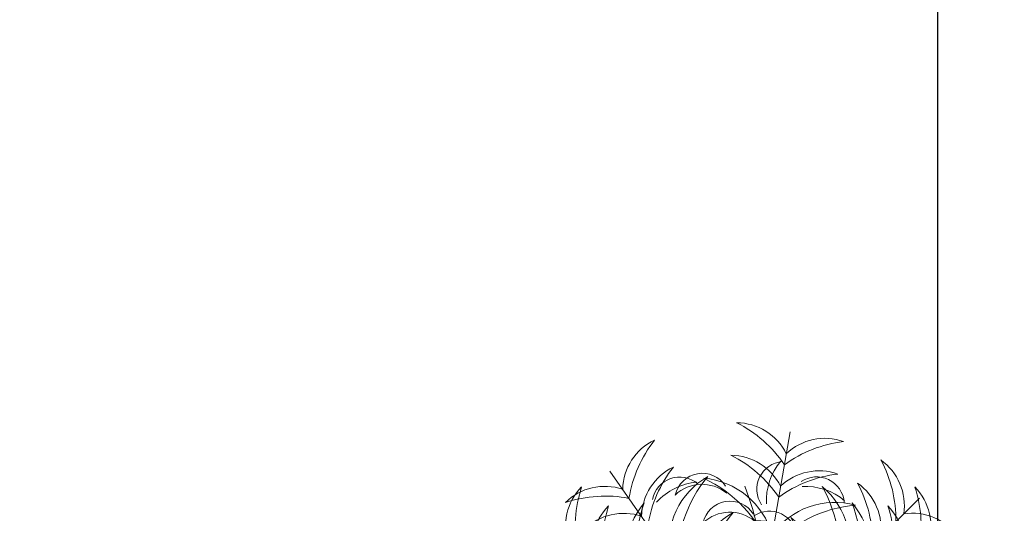
# Model space of a CAD drawing. Units: inches. Extents: x -48 to 50072, y 0 to 21068.
# Tile 30 of 75: x 415 to 467, y 327 to 353. Entities that reach past the tile are written whole.
import ezdxf

# ---------------------------------------------------------------- set-up
doc = ezdxf.new("R2010")
doc.units = ezdxf.units.IN
doc.header["$MEASUREMENT"] = 0
doc.layers.add('A-ANNO-DIMS', color=2, linetype='Continuous', lineweight=18)
doc.layers.add('L-PLNT', color=94, linetype='Continuous', lineweight=13)
doc.styles.get("Standard").update_dxf_attribs({"font": 'arial.ttf'})
doc.dimstyles.get("Standard").update_dxf_attribs({"dimtxt": 8, "dimasz": 0.18, "dimexe": 0.18, "dimexo": 0.0625, "dimgap": 0.09, "dimtad": 0, "dimtih": 1, "dimtoh": 1, "dimdec": 1, "dimzin": 0, "dimdsep": 46, "dimlunit": 4, "dimtxsty": 'Standard', "dimblk": 'ARCHTICK', "dimcen": 0.09, "dimadec": 0, "dimazin": 0, "dimtfac": 1, "dimtdec": 1, "dimtofl": 0, "dimtmove": 0, "dimatfit": 3, "dimldrblk": 'ARCHTICK', "dimfxl": 1, "dimtolj": 1, "dimtzin": 0, "dimarcsym": 0})

# ---------------------------------------------------------------- blocks, each defined once
blk = doc.blocks.new('A$C5D061C3B')
for p, q in [((3.377, 6.679), (3.377, 3.377)), ((1.483, 6.082), (3.377, 3.377)), ((5.259, 6.086), (3.365, 3.381)), ((1.03, 5.716), (3.365, 3.381)), ((5.712, 5.712), (3.377, 3.377)), ((0.125, 3.951), (3.377, 3.377)), ((6.629, 3.951), (3.377, 3.377)), ((0.66, 1.487), (3.365, 3.381)), ((1.483, 0.672), (3.377, 3.377)), ((6.07, 1.487), (3.365, 3.381)), ((3.951, 0.125), (3.377, 3.377)), ((6.082, 1.483), (3.377, 3.377))]:
    blk.add_line(p, q)
for centre, radius, start, end in [((2.763, 5.924), 0.762, 36.29, 99.6243), ((2.145, 5.032), 1.715, 44.0763, 73.3794), ((3.991, 5.924), 0.762, 80.3757, 143.71), ((4.61, 5.032), 1.715, 106.6206, 135.9237), ((2.419, 5.816), 0.762, 115.3757, 178.71), ((3.438, 5.44), 1.715, 141.6206, 170.9237), ((3.901, 5.939), 0.762, 125.3757, 188.71), ((4.969, 5.745), 1.715, 151.6206, 180.9237), ((3.305, 5.444), 1.715, 9.0763, 38.3794), ((4.323, 5.82), 0.762, 1.29, 64.6243), ((1.998, 5.617), 0.762, 125.3757, 188.71), ((3.066, 5.423), 1.715, 151.6206, 180.9237), ((2.763, 5.474), 0.762, 36.29, 99.6243), ((2.145, 4.581), 1.715, 44.0763, 73.3794), ((3.991, 5.474), 0.762, 80.3757, 143.71), ((4.61, 4.581), 1.715, 106.6206, 135.9237), ((3.871, 5.832), 0.38, 94.742, 213.7475), ((4.447, 5.681), 0.826, 139.618, 183.2106), ((4.744, 5.613), 0.762, 351.29, 54.6243), ((3.676, 5.419), 1.715, 359.0763, 28.3794), ((2.678, 5.447), 0.762, 115.3757, 178.71), ((3.696, 5.07), 1.715, 141.6206, 170.9237), ((4.064, 5.451), 0.762, 1.29, 64.6243), ((3.046, 5.075), 1.715, 9.0763, 38.3794), ((2.317, 5.298), 0.762, 125.3757, 188.71), ((3.385, 5.104), 1.715, 151.6206, 180.9237), ((3.344, 5.089), 1.056, 119.6063, 189.7511), ((4.177, 4.869), 1.77, 139.9634, 183.6288), ((3.398, 5.094), 1.056, 350.2489, 60.3937), ((2.565, 4.873), 1.77, 356.3712, 40.0366), ((1.413, 5.111), 0.762, 71.29, 134.6243), ((3.035, 5.062), 1.056, 129.6063, 199.7511), ((3.894, 4.989), 1.77, 149.9634, 193.6288), ((2.422, 4.799), 1.056, 25.2489, 95.3937), ((1.866, 4.14), 1.77, 31.3712, 75.0366), ((4.332, 4.799), 1.056, 84.6063, 154.7511), ((4.888, 4.14), 1.77, 104.9634, 148.6288), ((2.848, 4.985), 1.77, 346.3712, 30.0366), ((3.707, 5.058), 1.056, 340.2489, 50.3937), ((3.357, 5.1), 1.715, 359.0763, 28.3794), ((4.425, 5.294), 0.762, 351.29, 54.6243), ((1.419, 4.026), 1.715, 79.0763, 108.3794), ((1.991, 5.462), 0.38, 139.742, 258.7475), ((2.505, 5.763), 0.826, 184.618, 228.2106), ((3.688, 4.597), 1.056, 119.6063, 189.7511), ((4.522, 4.377), 1.77, 139.9634, 183.6288), ((2.221, 4.381), 1.77, 356.3712, 40.0366), ((3.054, 4.602), 1.056, 350.2489, 60.3937), ((5.564, 4.807), 0.762, 80.3757, 143.71), ((6.182, 3.914), 1.715, 106.6206, 135.9237), ((1.13, 4.748), 0.762, 81.29, 144.6243), ((1.324, 3.68), 1.715, 89.0763, 118.3794), ((1.671, 4.742), 0.762, 71.29, 134.6243), ((3.46, 4.637), 1.056, 129.6063, 199.7511), ((4.319, 4.565), 1.77, 149.9634, 193.6288), ((3.283, 4.633), 1.056, 340.2489, 50.3937), ((2.424, 4.56), 1.77, 346.3712, 30.0366), ((5.071, 4.746), 0.762, 45.3757, 108.71), ((5.419, 3.676), 1.715, 61.6206, 90.9237), ((5.613, 4.744), 0.762, 35.3757, 98.71), ((1.677, 3.657), 1.715, 79.0763, 108.3794), ((2.422, 4.198), 1.056, 25.2489, 95.3937), ((1.866, 3.54), 1.77, 31.3712, 75.0366), ((4.332, 4.198), 1.056, 84.6063, 154.7511), ((4.888, 3.54), 1.77, 104.9634, 148.6288), ((5.065, 3.661), 1.715, 71.6206, 100.9237), ((1.448, 4.43), 0.762, 81.29, 144.6243), ((3.868, 4.321), 1.029, 121.3654, 221.5741), ((4.556, 4.237), 1.557, 141.8122, 203.3335), ((4.035, 4.215), 1.029, 111.3654, 211.5741), ((2.707, 4.219), 1.029, 328.4259, 68.6346), ((2.044, 4.017), 1.557, 346.6665, 48.1878), ((4.698, 4.013), 1.557, 131.8122, 193.3335), ((2.187, 4.233), 1.557, 336.6665, 38.1878), ((2.875, 4.316), 1.029, 318.4259, 58.6346), ((5.294, 4.425), 0.762, 35.3757, 98.71), ((1.642, 3.362), 1.715, 89.0763, 118.3794), ((1.78, 3.994), 1.056, 60.2489, 130.3937), ((4.963, 3.998), 1.056, 49.6063, 119.7511), ((5.1, 3.357), 1.715, 61.6206, 90.9237), ((2.143, 4.564), 1.056, 164.6063, 234.7511), ((1.702, 3.136), 1.77, 66.3712, 110.0366), ((2.888, 4.998), 1.77, 184.9634, 228.6288), ((3.25, 4.435), 1.029, 156.3654, 256.5741), ((3.862, 4.761), 1.557, 176.8122, 238.3335), ((2.893, 4.761), 1.557, 301.6665, 3.1878), ((3.504, 4.435), 1.029, 283.4259, 23.6346), ((5.04, 3.14), 1.77, 69.9634, 113.6288), ((3.866, 4.998), 1.77, 311.3712, 355.0366), ((4.611, 4.564), 1.056, 305.2489, 15.3937), ((1.685, 3.712), 1.056, 70.2489, 140.3937), ((2.734, 4.46), 1.056, 164.6063, 234.7511), ((3.48, 4.893), 1.77, 184.9634, 228.6288), ((2.358, 3.686), 1.029, 3.4259, 103.6346), ((4.397, 3.686), 1.029, 76.3654, 176.5741), ((3.275, 4.893), 1.77, 311.3712, 355.0366), ((4.02, 4.46), 1.056, 305.2489, 15.3937), ((5.058, 3.707), 1.056, 39.6063, 109.7511), ((0.975, 4.424), 0.762, 160.3757, 223.71), ((1.962, 4.878), 1.715, 186.6206, 215.9237), ((1.419, 4.346), 0.762, 160.3757, 223.71), ((2.405, 4.8), 1.715, 186.6206, 215.9237), ((1.12, 4.31), 0.38, 94.742, 213.7475), ((1.696, 4.159), 0.826, 139.618, 183.2106), ((1.757, 2.853), 1.77, 76.3712, 120.0366), ((1.93, 3.14), 1.557, 21.6665, 83.1878), ((4.824, 3.14), 1.557, 96.8122, 158.3335), ((4.985, 2.848), 1.77, 59.9634, 103.6288), ((4.349, 4.8), 1.715, 324.0763, 353.3794), ((5.335, 4.346), 0.762, 316.29, 19.6243), ((4.793, 4.878), 1.715, 324.0763, 353.3794), ((5.779, 4.424), 0.762, 316.29, 19.6243), ((2.124, 3.502), 1.056, 60.2489, 130.3937), ((4.618, 3.506), 1.056, 49.6063, 119.7511), ((4.988, 5.812), 1.715, 279.0763, 308.3794), ((5.365, 4.794), 0.762, 271.29, 334.6243), ((2.109, 3.287), 1.056, 70.2489, 140.3937), ((2.046, 2.644), 1.77, 66.3712, 110.0366), ((2.387, 3.752), 0.574, 99.9865, 199.4034), ((3.599, 3.314), 1.651, 142.5759, 170.8942), ((4.696, 2.648), 1.77, 69.9634, 113.6288), ((4.633, 3.283), 1.056, 39.6063, 109.7511), ((2.182, 2.428), 1.77, 76.3712, 120.0366), ((4.56, 2.424), 1.77, 59.9634, 103.6288), ((1.588, 3.666), 0.38, 94.742, 213.7475), ((2.165, 3.515), 0.826, 139.618, 183.2106), ((2.365, 3.045), 1.029, 38.4259, 138.6346), ((2.84, 3.739), 0.372, 69.2257, 210.1279), ((3.109, 3.59), 0.515, 105.4398, 183.6694), ((4.377, 3.05), 1.029, 41.3654, 141.5741), ((2.426, 2.879), 1.029, 48.4259, 148.6346), ((2.328, 2.353), 1.557, 56.6665, 118.1878), ((4.414, 2.358), 1.557, 61.8122, 123.3335), ((4.316, 2.875), 1.029, 31.3654, 131.5741), ((0.762, 3.214), 0.762, 116.29, 179.6243), ((1.534, 2.451), 1.715, 124.0763, 153.3794), ((1.206, 3.136), 0.762, 116.29, 179.6243), ((1.977, 2.373), 1.715, 124.0763, 153.3794), ((1.062, 4.452), 0.826, 229.618, 273.2106), ((0.91, 3.875), 0.38, 184.742, 303.7475), ((4.777, 2.373), 1.715, 26.6206, 55.9237), ((5.549, 3.136), 0.762, 0.3757, 63.71), ((1.811, 2.684), 1.056, 105.2489, 175.3937), ((2.363, 2.022), 1.77, 111.3712, 155.0366), ((2.51, 2.191), 1.557, 66.6665, 128.1878), ((2.729, 4.702), 1.557, 221.8122, 283.3335), ((2.527, 4.039), 1.029, 201.3654, 301.5741), ((4.233, 2.187), 1.557, 51.8122, 113.3335), ((4.001, 4.702), 1.557, 256.6665, 318.1878), ((4.013, 4.698), 1.557, 256.6665, 318.1878), ((4.203, 4.039), 1.029, 238.4259, 338.6346), ((4.215, 4.035), 1.029, 238.4259, 338.6346), ((4.391, 2.022), 1.77, 24.9634, 68.6288), ((4.943, 2.684), 1.056, 4.6063, 74.7511), ((6.053, 3.533), 0.38, 146.2525, 265.258), ((6.629, 3.684), 0.826, 176.7894, 220.382), ((2.185, 0.015), 3.567, 70.4772, 111.6585), ((2.403, 2.58), 1.056, 105.2489, 175.3937), ((2.955, 1.917), 1.77, 111.3712, 155.0366), ((2.007, 3.071), 0.506, 93.8744, 233.9763), ((2.489, 2.932), 0.825, 128.7536, 199.097), ((2.903, 2.8), 0.855, 116.4477, 194.3672), ((4.744, 1.779), 2.789, 140.4007, 163.139), ((2.741, 3.253), 0.372, 114.2257, 255.1279), ((3.037, 3.338), 0.515, 150.4398, 228.6694), ((3.799, 1.917), 1.77, 24.9634, 68.6288), ((4.352, 2.58), 1.056, 4.6063, 74.7511), ((5.935, 2.842), 0.762, 35.3757, 98.71), ((1.447, 3.129), 0.376, 122.0577, 257.8533), ((1.751, 3.126), 0.529, 140.1845, 223.654), ((4.912, 0.157), 3.567, 115.4772, 156.6585), ((2.896, 2.427), 1.029, 83.4259, 183.6346), ((3.359, 1.911), 1.557, 101.6665, 163.1878), ((6.727, 2.189), 3.567, 160.4772, 201.6585), ((3.395, 1.911), 1.557, 16.8122, 78.3335), ((3.858, 2.427), 1.029, 356.3654, 96.5741), ((5.741, 1.774), 1.715, 61.6206, 90.9237), ((2.412, 2.943), 0.574, 144.9865, 244.4034), ((3.578, 3.49), 1.651, 187.5759, 215.8942), ((2.145, 3.693), 1.056, 209.6063, 279.7511), ((2.365, 4.526), 1.77, 229.9634, 273.6288), ((2.328, 4.401), 1.557, 241.8122, 303.3335), ((3.697, 2.369), 1.029, 128.4259, 228.6346), ((4.389, 2.332), 1.557, 146.6665, 208.1878), ((4.698, 2.741), 1.557, 166.6665, 228.1878), ((2.341, 2.332), 1.557, 331.8122, 33.3335), ((2.353, 2.328), 1.557, 331.8122, 33.3335), ((3.033, 2.369), 1.029, 311.3654, 51.5741), ((3.045, 2.365), 1.029, 311.3654, 51.5741), ((4.365, 4.526), 1.77, 266.3712, 310.0366), ((4.377, 4.522), 1.77, 266.3712, 310.0366), ((4.585, 3.693), 1.056, 260.2489, 330.3937), ((4.597, 3.688), 1.056, 260.2489, 330.3937), ((1.067, 2.749), 0.376, 122.0577, 257.8533), ((1.37, 2.745), 0.529, 140.1845, 223.654), ((2.365, 3.709), 1.029, 221.3654, 321.5741), ((1.911, 3.359), 1.557, 286.8122, 348.3335), ((2.427, 2.896), 1.029, 266.3654, 6.5741), ((3.003, 2.844), 0.372, 159.2257, 300.1279), ((3.152, 3.113), 0.515, 195.4398, 273.6694), ((4.035, 2.539), 1.029, 148.4259, 248.6346), ((4.435, 3.25), 1.029, 193.4259, 293.6346), ((4.761, 3.862), 1.557, 211.6665, 273.1878), ((1.873, 4.181), 1.77, 229.9634, 273.6288), ((1.653, 3.348), 1.056, 209.6063, 279.7511), ((3.45, 2.634), 0.855, 161.4477, 239.3672), ((5.474, 3.214), 2.789, 185.4007, 208.139), ((4.857, 4.181), 1.77, 266.3712, 310.0366), ((5.077, 3.348), 1.056, 260.2489, 330.3937), ((4.099, 2.051), 1.77, 156.3712, 200.0366), ((2.632, 2.051), 1.77, 339.9634, 23.6288), ((2.644, 2.046), 1.77, 339.9634, 23.6288), ((4.869, 4.177), 1.77, 266.3712, 310.0366), ((5.089, 3.344), 1.056, 260.2489, 330.3937), ((1.122, 2.441), 0.38, 139.742, 258.7475), ((1.636, 2.741), 0.826, 184.618, 228.2106), ((1.908, 2.317), 0.38, 139.742, 258.7475), ((3.24, 2.128), 1.056, 150.2489, 220.3937), ((4.963, 4.749), 2.789, 230.4007, 253.139), ((3.49, 2.128), 1.056, 319.6063, 29.7511), ((3.502, 2.124), 1.056, 319.6063, 29.7511), ((6.244, 3.948), 1.715, 234.0763, 263.3794), ((2.046, 4.111), 1.77, 249.9634, 293.6288), ((2.124, 3.252), 1.056, 229.6063, 299.7511), ((2.422, 2.617), 0.826, 184.618, 228.2106), ((2.624, 2.192), 0.506, 138.8744, 278.9763), ((3.064, 2.435), 0.825, 173.7536, 244.097), ((4.522, 2.378), 1.77, 176.3712, 220.0366), ((3.942, 2.908), 0.855, 206.4477, 284.3672), ((1.672, 3.7), 1.715, 231.6206, 260.9237), ((1.295, 2.682), 0.762, 205.3757, 268.71), ((2.748, 1.784), 1.056, 150.2489, 220.3937), ((3.607, 1.706), 1.77, 156.3712, 200.0366), ((3.428, 3.603), 1.651, 232.5759, 260.8942), ((2.99, 2.391), 0.574, 189.9865, 289.4034), ((3.688, 2.157), 1.056, 170.2489, 240.3937), ((1.917, 2.955), 1.77, 294.9634, 338.6288), ((4.893, 3.48), 1.77, 221.3712, 265.0366), ((3.124, 1.706), 1.77, 339.9634, 23.6288), ((3.136, 1.702), 1.77, 339.9634, 23.6288), ((3.982, 1.784), 1.056, 319.6063, 29.7511), ((3.994, 1.78), 1.056, 319.6063, 29.7511), ((5.79, 2.962), 0.762, 226.29, 289.6243), ((5.058, 3.7), 1.715, 279.0763, 308.3794), ((5.07, 3.696), 1.715, 279.0763, 308.3794), ((5.435, 2.682), 0.762, 271.29, 334.6243), ((5.447, 2.678), 0.762, 271.29, 334.6243), ((0.926, 2.424), 0.762, 205.3757, 268.71), ((1.303, 3.442), 1.715, 231.6206, 260.9237), ((2.58, 2.403), 1.056, 274.6063, 344.7511), ((4.46, 2.734), 1.056, 215.2489, 285.3937), ((5.427, 3.442), 1.715, 279.0763, 308.3794), ((5.44, 3.438), 1.715, 279.0763, 308.3794), ((5.804, 2.424), 0.762, 271.29, 334.6243), ((5.816, 2.419), 0.762, 271.29, 334.6243), ((1.702, 3.619), 1.77, 249.9634, 293.6288), ((1.78, 2.76), 1.056, 229.6063, 299.7511), ((2, 1.676), 0.762, 161.29, 224.6243), ((3.086, 1.681), 1.715, 169.0763, 198.3794), ((2.188, 1.837), 0.376, 167.0577, 302.8533), ((2.405, 2.049), 0.529, 185.1845, 268.654), ((4.177, 1.886), 1.77, 176.3712, 220.0366), ((3.81, 2.493), 0.825, 218.7536, 289.097), ((3.671, 2.011), 0.506, 183.8744, 323.9763), ((5.385, 1.584), 0.38, 101.2525, 220.258), ((5.899, 1.283), 0.826, 131.7894, 175.382), ((3.645, 1.681), 1.715, 341.6206, 10.9237), ((4.73, 1.676), 0.762, 315.3757, 18.71), ((3.657, 1.677), 1.715, 341.6206, 10.9237), ((4.742, 1.671), 0.762, 315.3757, 18.71), ((3.344, 1.665), 1.056, 170.2489, 240.3937), ((1.631, 1.417), 0.762, 161.29, 224.6243), ((2.717, 1.423), 1.715, 169.0763, 198.3794), ((2.022, 2.363), 1.77, 294.9634, 338.6288), ((4.998, 2.888), 1.77, 221.3712, 265.0366), ((4.014, 1.423), 1.715, 341.6206, 10.9237), ((5.099, 1.417), 0.762, 315.3757, 18.71), ((3.227, 2.169), 0.826, 229.618, 273.2106), ((3.076, 1.593), 0.38, 184.742, 303.7475), ((2.684, 1.811), 1.056, 274.6063, 344.7511), ((4.564, 2.143), 1.056, 215.2489, 285.3937), ((5.808, 1.754), 1.715, 189.0763, 218.3794), ((1.671, 2.012), 0.762, 225.3757, 288.71), ((1.677, 3.098), 1.715, 251.6206, 280.9237), ((2.188, 1.299), 0.376, 167.0577, 302.8533), ((2.405, 1.511), 0.529, 185.1845, 268.654), ((3.696, 1.684), 1.715, 189.0763, 218.3794), ((3.616, 1.755), 0.529, 230.1845, 313.654), ((3.613, 1.452), 0.376, 212.0577, 347.8533), ((4.79, 1.377), 0.762, 181.29, 244.6243), ((2.678, 1.307), 0.762, 181.29, 244.6243), ((1.419, 2.729), 1.715, 251.6206, 280.9237), ((1.413, 1.643), 0.762, 225.3757, 288.71), ((2.432, 1.124), 0.38, 184.742, 303.7475), ((3.438, 1.315), 1.715, 189.0763, 218.3794), ((2.583, 1.701), 0.826, 229.618, 273.2106), ((2.373, 1.977), 1.715, 296.6206, 325.9237), ((3.528, 0.69), 0.38, 56.2525, 175.258), ((3.997, 1.374), 0.529, 230.1845, 313.654), ((3.994, 1.071), 0.376, 212.0577, 347.8533), ((4.8, 2.405), 1.715, 234.0763, 263.3794), ((2.419, 0.938), 0.762, 181.29, 244.6243), ((3.136, 1.206), 0.762, 270.3757, 333.71), ((3.68, 0.113), 0.826, 86.7894, 130.382), ((4.346, 1.419), 0.762, 226.29, 289.6243), ((2.451, 1.534), 1.715, 296.6206, 325.9237), ((4.878, 1.962), 1.715, 234.0763, 263.3794), ((3.214, 0.762), 0.762, 270.3757, 333.71), ((4.424, 0.975), 0.762, 226.29, 289.6243)]:
    blk.add_arc(centre, radius, start, end)
blk = doc.blocks.new('_ArchTick')
at = {"color": 0, "linetype": 'ByBlock', "const_width": 0.15}
blk.add_lwpolyline([(-0.5, -0.5), (0.5, 0.5)], dxfattribs=at)
blk = doc.blocks.new('*D118')
at = {"layer": 'A-ANNO-DIMS', "color": 0, "lineweight": -2, "transparency": 16777216}
for p, q in [((297.017, 488.712), (297.017, 165.945)), ((463.517, 488.712), (463.517, 165.945)), ((297.017, 166.125), (367.026, 166.125)), ((463.517, 166.125), (393.509, 166.125))]:
    blk.add_line(p, q, dxfattribs=at)
at = {"layer": 'Defpoints', "color": 0, "transparency": 16777216}
for p in [(297.017, 488.775), (463.517, 488.775), (463.517, 166.125)]:
    blk.add_point(p, dxfattribs=at)
at = {"layer": 'A-ANNO-DIMS', "color": 0, "lineweight": -2, "transparency": 16777216, "xscale": 0.18, "yscale": 0.18, "zscale": 0.18, "rotation": 180}
blk.add_blockref('_ArchTick', (297.017, 166.125), dxfattribs=at)
at = {"layer": 'A-ANNO-DIMS', "color": 0, "lineweight": -2, "transparency": 16777216, "xscale": 0.18, "yscale": 0.18, "zscale": 0.18}
blk.add_blockref('_ArchTick', (463.517, 166.125), dxfattribs=at)
at = {"layer": 'A-ANNO-DIMS', "color": 0, "transparency": 16777216, "insert": (380.267, 166.125), "char_height": 8, "attachment_point": 5}
blk.add_mtext('\\A1;166.5', dxfattribs=at)
blk = doc.blocks.new('*D119')
at = {"layer": 'A-ANNO-DIMS', "color": 0, "lineweight": -2, "transparency": 16777216}
for p, q in [((463.517, 451.012), (463.517, 165.945)), ((549.017, 451.012), (549.017, 165.945)), ((463.517, 166.125), (495.752, 166.125)), ((549.017, 166.125), (516.783, 166.125))]:
    blk.add_line(p, q, dxfattribs=at)
at = {"layer": 'Defpoints', "color": 0, "transparency": 16777216}
for p in [(463.517, 451.075), (549.017, 451.075), (549.017, 166.125)]:
    blk.add_point(p, dxfattribs=at)
at = {"layer": 'A-ANNO-DIMS', "color": 0, "lineweight": -2, "transparency": 16777216, "xscale": 0.18, "yscale": 0.18, "zscale": 0.18, "rotation": 180}
blk.add_blockref('_ArchTick', (463.517, 166.125), dxfattribs=at)
at = {"layer": 'A-ANNO-DIMS', "color": 0, "lineweight": -2, "transparency": 16777216, "xscale": 0.18, "yscale": 0.18, "zscale": 0.18}
blk.add_blockref('_ArchTick', (549.017, 166.125), dxfattribs=at)
at = {"layer": 'A-ANNO-DIMS', "color": 0, "transparency": 16777216, "insert": (506.267, 166.125), "char_height": 8, "attachment_point": 5}
blk.add_mtext('\\A1;85.5', dxfattribs=at)

msp = doc.modelspace()

# ---------------------------------------------------------------- block references
at = {"layer": 'L-PLNT', "xscale": 3.862191520948588, "yscale": 3.862191520948588, "zscale": 3.862191520948588, "rotation": 270}
msp.add_blockref('A$C5D061C3B', (440.483, 331.436), dxfattribs=at)

# ---------------------------------------------------------------- dimensions: what is measured, and where the dimension line sits
at = {"layer": 'A-ANNO-DIMS'}
for base, p1, p2, picture, middle in [((463.517, 166.125), (297.017, 488.775), (463.517, 488.775), '*D118', (380.267, 166.125)), ((549.017, 166.125), (463.517, 451.075), (549.017, 451.075), '*D119', (506.267, 166.125))]:
    dim = msp.add_linear_dim(base=base, p1=p1, p2=p2, dimstyle='Standard', override={"dimdec": 1, "dimlfac": 1, "dimrnd": 0, "dimzin": 0, "dimdsep": 46, "dimlunit": 2}, dxfattribs=at)
    dim.commit()
    dim.dimension.update_dxf_attribs({"geometry": picture, "text_midpoint": middle})

doc.saveas('drawing.dxf')
